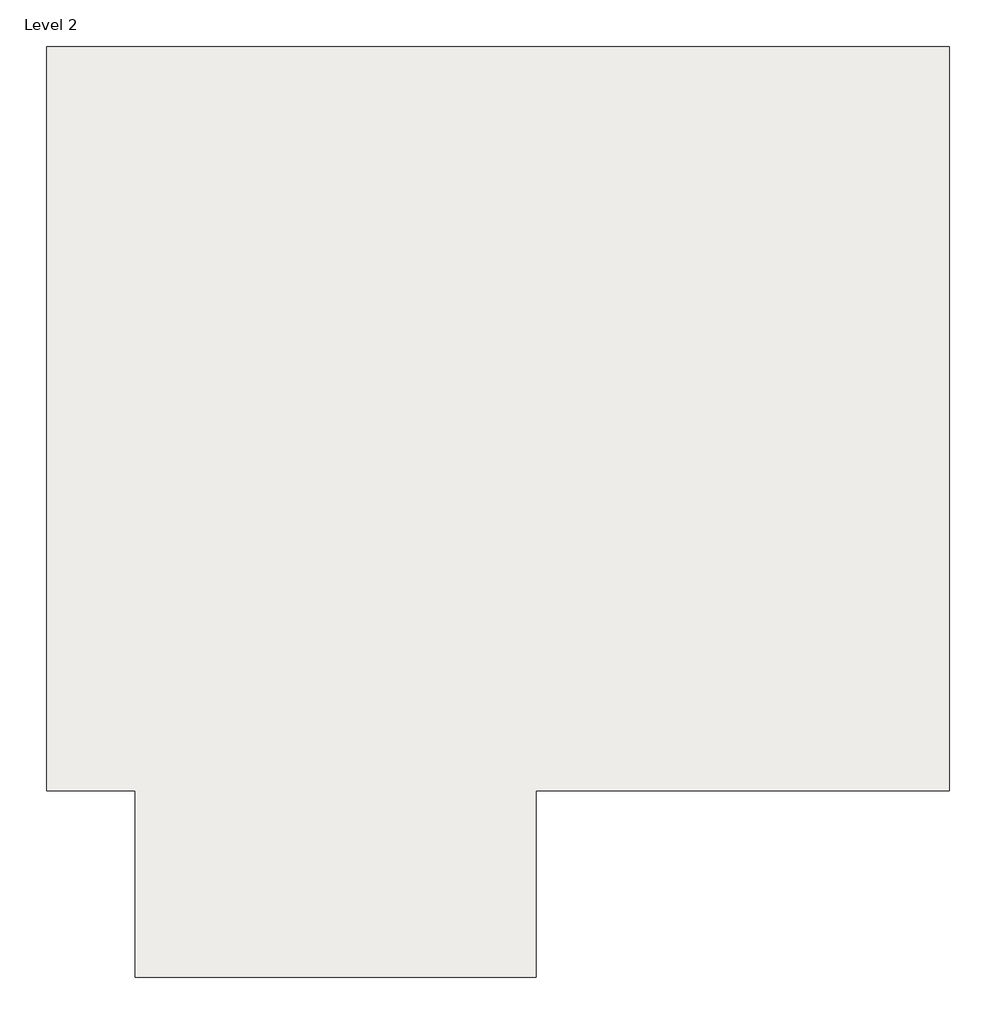
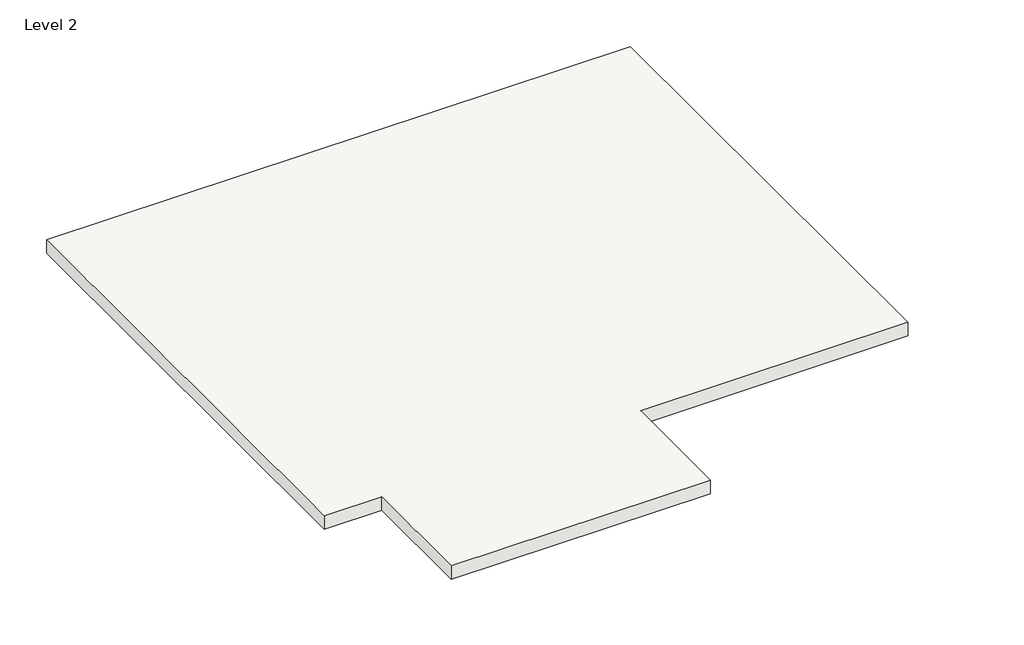
# One storey: 1 roof.
"""IFC4 building model written with IfcOpenShell, lengths in millimetres."""

from ifc_helpers import new_model, si_unit, frame, origin, place, context, project, spatial, polyline, outline, extrude, element, save

model = new_model("IFC4")

# Units and contexts
model_context = context("Model", 3, world=origin())
ifc_project = project(units=[si_unit("LENGTHUNIT", "METRE", prefix="MILLI")], contexts=[model_context])

# Site, building, storey
site = spatial("IfcSite", under=ifc_project)
building = spatial("IfcBuilding", under=site)
storey = spatial("IfcBuildingStorey", under=building, Name="Level 2", Elevation=3048.0)

# Roof
placement = place(None, origin())
element("IfcRoof", 1, ObjectType="Generic - 12\"", at=placement, inside=storey, context=model_context, shape_type="SweptSolid", body=[
    extrude(outline(polyline([(-13636.0402453, 12155.4116886), (-1215.4402453, 12155.4116886), (-1215.4402453, 1919.2116886), (-6905.0402453, 1919.2116886), (-6905.0402453, -646.1883114), (-12416.8402453, -646.1883114), (-12416.8402453, 1919.2116886), (-13636.0402453, 1919.2116886), (-13636.0402453, 12155.4116886)])), frame((0.0, 0.0, 3048.0), z_axis=(0.0, 0.0, 1.0), x_axis=(1.0, 0.0, 0.0)), (0.0, 0.0, 1.0), 304.8),
])

save(model, "model.ifc")

# Revit data of these elements
# Type "Generic - 12\""
#   Assembly Code = "B1020"
#   Layers, outside or top first: 1' - 0" "Brick, Soldier Course" (function 1)
# Element 1 (IfcRoof, "Generic - 12\"")
#   built-in parameter 1001705 = 11 (stored number, unit not read)
#   built-in parameter 1001710 = 33615
#   Phase Created = New Construction
#   Materials on its faces: "Brick, Soldier Course"
# Materials
#   "Brick, Soldier Course": class "Masonry", colour RGB 170 98 104, transparency 0, Description = "Common brick soldier coursed", Cost = 0
